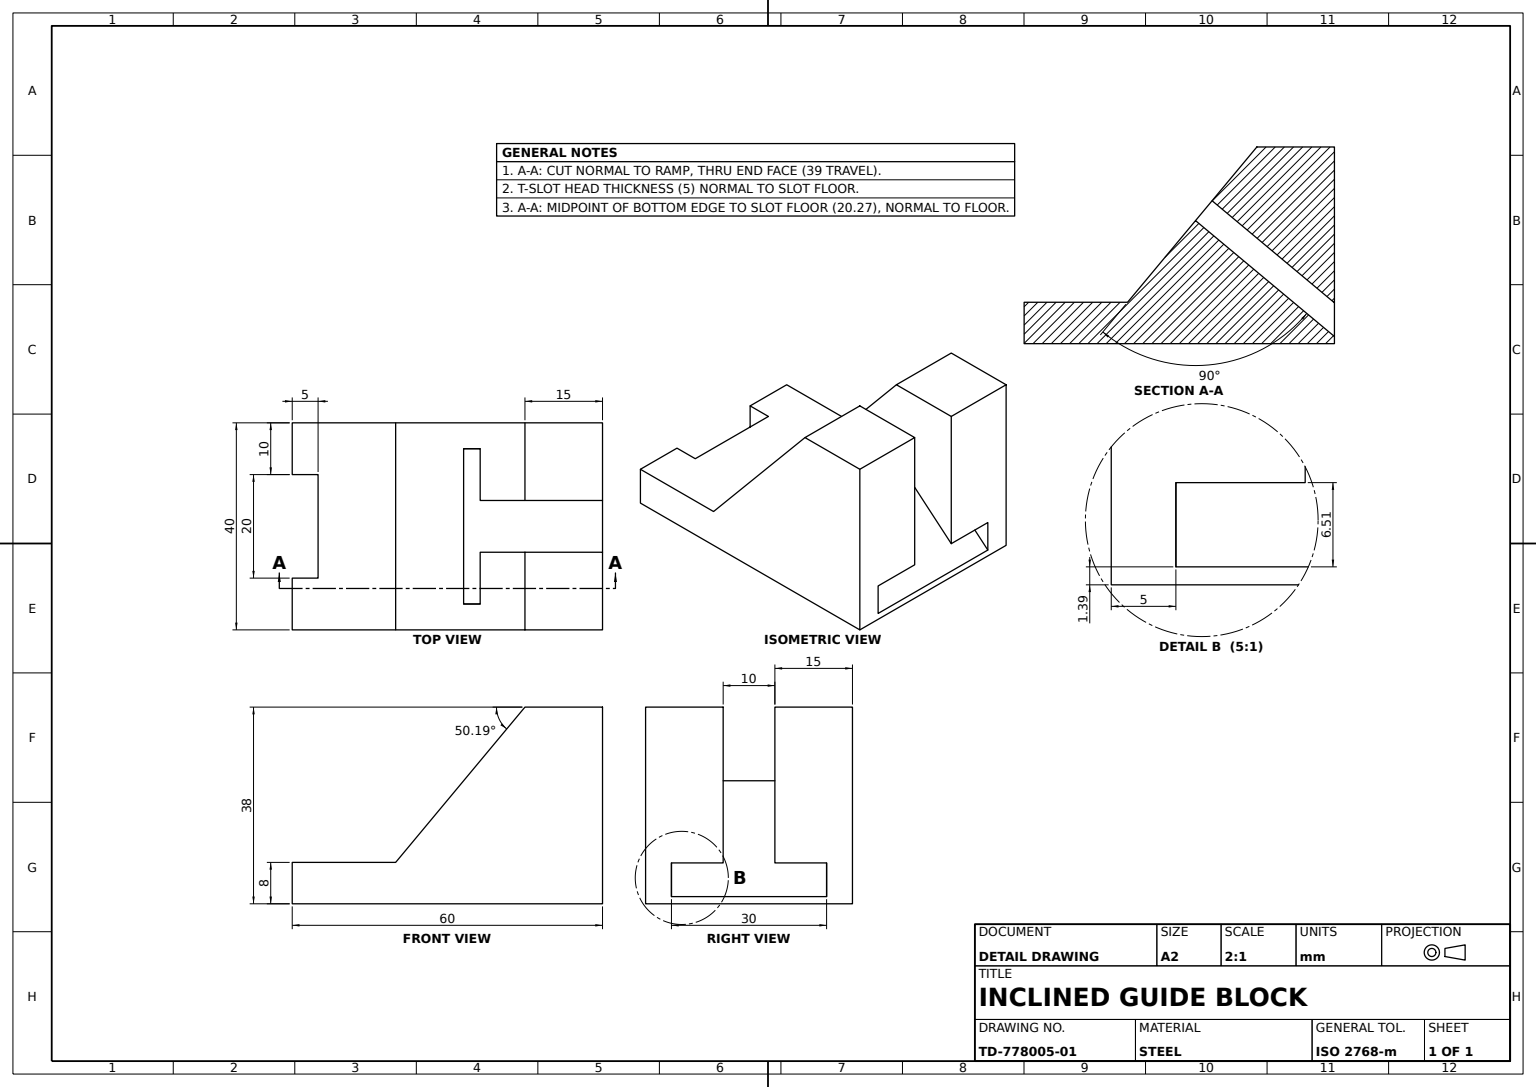
from build123d import *

# Parameters (mm, degrees)
BASE_PLATE_SKETCH_W                   = 40
BASE_PLATE_SKETCH_H                   = 60
BASE_PLATE_60X40X8_DEPTH              = 8
BASE_NOTCH_SKETCH_W                   = 20
BASE_NOTCH_SKETCH_H                   = 5
BASE_NOTCH_20X5_DEPTH                 = 20
UPRIGHT_BLOCK_SKETCH_W                = 40
UPRIGHT_BLOCK_SKETCH_H                = 30
UPRIGHT_BLOCK_40X30X40_DEPTH          = 40
SLOPED_FACE_CUT_DEPTH                 = 40
TOP_SLOT_CUT_DEPTH                    = 39
ANGLED_SLOT_THROUGH_SLOPED_FACE_REACH = 54.383
ANGLED_SLOT_SKETCH_W                  = 10
ANGLED_SLOT_SKETCH_H                  = 15


with BuildPart() as part:
    # Base Plate Sketch → Base Plate 60x40x8 (new body)
    with BuildSketch(Plane(origin=(0, 0, 0), x_dir=(1, 0, 0), z_dir=(0, 1, 0))):
        Rectangle(BASE_PLATE_SKETCH_W, BASE_PLATE_SKETCH_H)
    extrude(amount=BASE_PLATE_60X40X8_DEPTH)

    # Base Notch Sketch → Base Notch 20x5 (cut)
    with BuildSketch(Plane(origin=(0, 8, 0), x_dir=(1, 0, 0), z_dir=(0, 1, 0))):
        with Locations((0, -27.5)):
            Rectangle(BASE_NOTCH_SKETCH_W, BASE_NOTCH_SKETCH_H)
    extrude(amount=-BASE_NOTCH_20X5_DEPTH, mode=Mode.SUBTRACT)

    # Upright Block Sketch → Upright Block 40x30x40 (add)
    with BuildSketch(Plane(origin=(20, 0, 0), x_dir=(0, 0, -1), z_dir=(1, 0, 0))):
        with Locations((10, 23)):
            Rectangle(UPRIGHT_BLOCK_SKETCH_W, UPRIGHT_BLOCK_SKETCH_H)
    extrude(amount=-UPRIGHT_BLOCK_40X30X40_DEPTH)

    # Slope Cut Sketch → Sloped Face Cut (cut)
    with BuildSketch(Plane(origin=(20, 0, 0), x_dir=(0, 0, -1), z_dir=(1, 0, 0))):
        Polygon((15, 38), (-10, 38), (-10, 8), align=None)
    extrude(amount=-SLOPED_FACE_CUT_DEPTH, mode=Mode.SUBTRACT)

    # Top Slot Sketch → Top Slot Cut (cut)
    with BuildSketch(Plane(origin=(0, 8.196721311, 9.836065574), x_dir=(1, 0, 0), z_dir=(0, 0.6401843996644799, 0.768221279597376))):
        Polygon((-5, 25.272676797), (-15, 25.272676797), (-15, 20.272676797), (15, 20.272676797), (15, 25.272676797), (5, 25.272676797), (5, 38.79517462), (-5, 38.79517462), align=None)
    extrude(amount=-TOP_SLOT_CUT_DEPTH, mode=Mode.SUBTRACT)

    # Angled Slot Sketch → Angled Slot Through Sloped Face (cut, up to next)
    with BuildSketch(Plane(origin=(0, 38, 0), x_dir=(1, 0, 0), z_dir=(0, 1, 0)), mode=Mode.PRIVATE) as angled_slot_through_sloped_face_sk1:
        with Locations((0, 22.5)):
            Rectangle(ANGLED_SLOT_SKETCH_W, ANGLED_SLOT_SKETCH_H)
    angled_slot_through_sloped_face_tool1 = extrude(angled_slot_through_sloped_face_sk1.sketch, amount=-ANGLED_SLOT_THROUGH_SLOPED_FACE_REACH, mode=Mode.PRIVATE) & part.part
    add(angled_slot_through_sloped_face_tool1.solids().sort_by_distance((0, 38, -22.5))[0], mode=Mode.SUBTRACT)


solid = part.part
